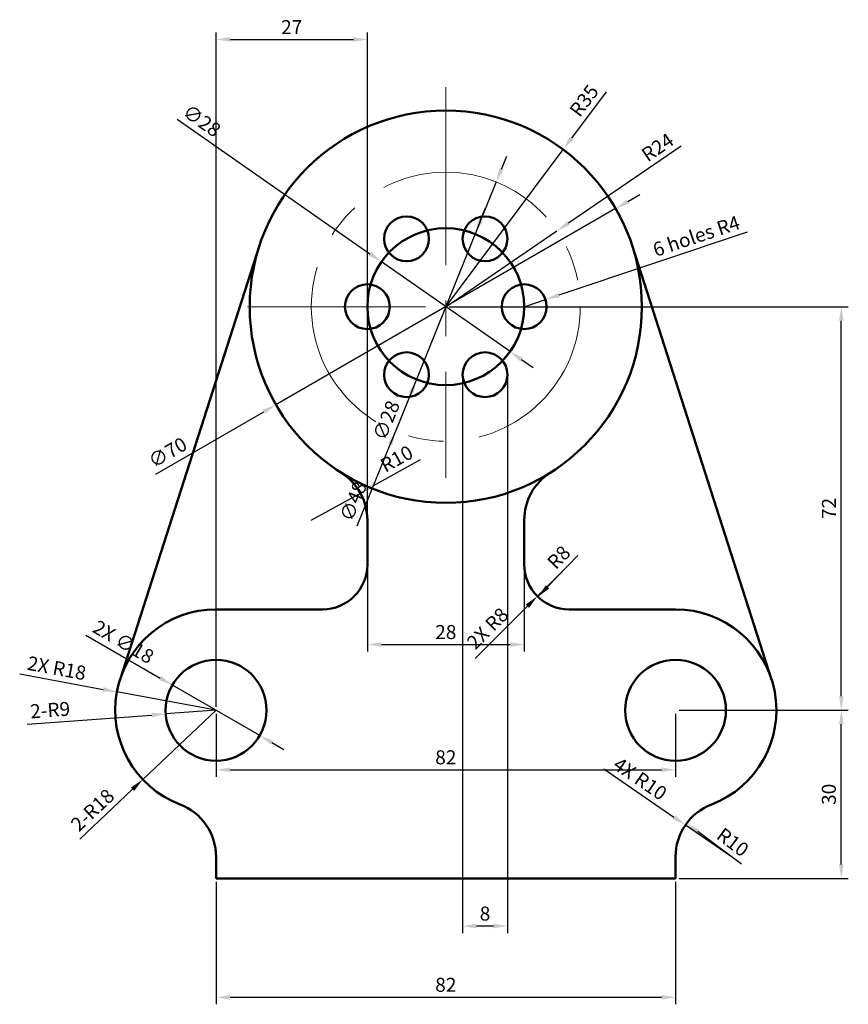
# Model space of a CAD drawing. Units: millimetres. Extents: x 2340 to 2488, y 1384 to 1560.
import ezdxf

# ---------------------------------------------------------------- set-up
doc = ezdxf.new("R2010")
doc.units = ezdxf.units.MM
doc.linetypes.add('CENTER', pattern=[50.8, 31.75, -6.35, 6.35, -6.35])
for name, color, linetype, lineweight in [('M-CNTR', 4, 'CENTER', 18), ('M-DIMS', 2, 'Continuous', 25), ('M-OUTL', 7, 'Continuous', 50)]:
    doc.layers.add(name, color=color, linetype=linetype, lineweight=lineweight)
doc.styles.get("Standard").update_dxf_attribs({"font": 'arial.ttf'})
doc.dimstyles.new('ISO-25', dxfattribs={"dimtxt": 2.5, "dimasz": 2.5, "dimexe": 1.25, "dimexo": 0.625, "dimtad": 1, "dimdec": 1, "dimdsep": 46, "dimtxsty": 'Standard', "dimcen": 2.5, "dimadec": 0, "dimazin": 0, "dimtfac": 1, "dimtdec": 1, "dimtmove": 0, "dimatfit": 3, "dimfxl": 1, "dimarcsym": 0})

# ---------------------------------------------------------------- blocks, each defined once
blk = doc.blocks.new('*U1')
blk.add_circle((0, 0), 4)
blk = doc.blocks.new('*U2')
at = {"layer": 'M-OUTL', "color": 0, "linetype": 'ByBlock', "lineweight": -2, "transparency": 16777216}
for p, rotation in [((2408.96, 1520.78), 300), ((2422.96, 1520.78), 239.9999999999999), ((2429.96, 1508.66), 180), ((2408.96, 1496.53), 59.99999999999999), ((2422.96, 1496.53), 119.9999999999999)]:
    blk.add_blockref('*U1', p, dxfattribs=dict(at, rotation=rotation))
blk.add_blockref('*U1', (2401.96, 1508.66), dxfattribs=at)
blk = doc.blocks.new('*D3')
at = {"layer": 'Defpoints', "color": 0, "lineweight": 100, "transparency": 16777216}
for p in [(2374.96, 1436.66), (2456.96, 1436.66), (2456.96, 1426.04)]:
    blk.add_point(p, dxfattribs=at)
at = {"layer": 'M-DIMS', "color": 0, "lineweight": -2, "transparency": 16777216}
for p, q in [((2374.96, 1436.03), (2374.96, 1424.79)), ((2456.96, 1436.03), (2456.96, 1424.79)), ((2377.46, 1426.04), (2454.46, 1426.04))]:
    blk.add_line(p, q, dxfattribs=at)
at = {"layer": 'M-DIMS', "color": 0, "lineweight": 100, "transparency": 16777216}
for points in [[(2377.46, 1426.46), (2377.46, 1425.63), (2374.96, 1426.04)], [(2454.46, 1426.46), (2454.46, 1425.63), (2456.96, 1426.04)]]:
    blk.add_solid(points, dxfattribs=at)
at = {"layer": 'M-DIMS', "color": 0, "transparency": 16777216, "insert": (2415.96, 1427.94), "char_height": 2.5, "attachment_point": 5}
blk.add_mtext('82', dxfattribs=at)
blk = doc.blocks.new('*D4')
at = {"layer": 'Defpoints', "color": 0, "lineweight": 100, "transparency": 16777216}
for p in [(2374.96, 1406.66), (2456.96, 1406.66), (2456.96, 1385.45)]:
    blk.add_point(p, dxfattribs=at)
at = {"layer": 'M-DIMS', "color": 0, "lineweight": -2, "transparency": 16777216}
for p, q in [((2374.96, 1406.03), (2374.96, 1384.2)), ((2456.96, 1406.03), (2456.96, 1384.2)), ((2377.46, 1385.45), (2454.46, 1385.45))]:
    blk.add_line(p, q, dxfattribs=at)
at = {"layer": 'M-DIMS', "color": 0, "lineweight": 100, "transparency": 16777216}
for points in [[(2377.46, 1385.86), (2377.46, 1385.03), (2374.96, 1385.45)], [(2454.46, 1385.86), (2454.46, 1385.03), (2456.96, 1385.45)]]:
    blk.add_solid(points, dxfattribs=at)
at = {"layer": 'M-DIMS', "color": 0, "transparency": 16777216, "insert": (2415.96, 1387.35), "char_height": 2.5, "attachment_point": 5}
blk.add_mtext('82', dxfattribs=at)
blk = doc.blocks.new('*D5')
at = {"layer": 'Defpoints', "color": 0, "lineweight": 100, "transparency": 16777216}
for p in [(2374.96, 1436.66), (2361.88, 1424.29)]:
    blk.add_point(p, dxfattribs=at)
at = {"layer": 'M-DIMS', "color": 0, "lineweight": -2, "transparency": 16777216}
for p, q in [((2374.96, 1436.66), (2361.88, 1424.29)), ((2350.62, 1413.64), (2360.07, 1422.57))]:
    blk.add_line(p, q, dxfattribs=at)
at = {"layer": 'M-DIMS', "color": 0, "lineweight": 100, "transparency": 16777216}
blk.add_solid([(2359.78, 1422.88), (2360.35, 1422.27), (2361.88, 1424.29)], dxfattribs=at)
at = {"layer": 'M-DIMS', "color": 0, "transparency": 16777216, "insert": (2353.13, 1418.63), "char_height": 2.5, "attachment_point": 5, "rotation": 43.3974}
blk.add_mtext('2-R18', dxfattribs=at)
blk = doc.blocks.new('*D6')
at = {"layer": 'Defpoints', "color": 0, "lineweight": 100, "transparency": 16777216}
for p in [(2365.99, 1436), (2374.96, 1436.66)]:
    blk.add_point(p, dxfattribs=at)
at = {"layer": 'M-DIMS', "color": 0, "lineweight": -2, "transparency": 16777216}
for p, q in [((2341.24, 1434.17), (2363.49, 1435.81)), ((2374.96, 1436.66), (2365.99, 1436))]:
    blk.add_line(p, q, dxfattribs=at)
at = {"layer": 'M-DIMS', "color": 0, "lineweight": 100, "transparency": 16777216}
blk.add_solid([(2363.46, 1436.23), (2363.52, 1435.4), (2365.99, 1436)], dxfattribs=at)
at = {"layer": 'M-DIMS', "color": 0, "transparency": 16777216, "insert": (2345.37, 1436.38), "char_height": 2.5, "attachment_point": 5, "rotation": 4.2165}
blk.add_mtext('2-R9', dxfattribs=at)
blk = doc.blocks.new('*D7')
at = {"layer": 'Defpoints', "color": 0, "lineweight": 100, "transparency": 16777216}
for p in [(2458.96, 1416.5), (2466.96, 1410.51)]:
    blk.add_point(p, dxfattribs=at)
at = {"layer": 'M-DIMS', "color": 0, "lineweight": -2, "transparency": 16777216}
blk.add_line((2468.74, 1409.18), (2460.96, 1415), dxfattribs=at)
at = {"layer": 'M-DIMS', "color": 0, "lineweight": 100, "transparency": 16777216}
blk.add_solid([(2461.21, 1415.33), (2460.71, 1414.67), (2458.96, 1416.5)], dxfattribs=at)
at = {"layer": 'M-DIMS', "color": 0, "transparency": 16777216, "insert": (2466.99, 1412.86), "char_height": 2.5, "attachment_point": 5, "rotation": 323.1905}
blk.add_mtext('R10', dxfattribs=at)
blk = doc.blocks.new('*D8')
at = {"layer": 'Defpoints', "color": 0, "lineweight": 100, "transparency": 16777216}
for p in [(2437.96, 1462.66), (2432.41, 1456.9)]:
    blk.add_point(p, dxfattribs=at)
at = {"layer": 'M-DIMS', "color": 0, "lineweight": -2, "transparency": 16777216}
blk.add_line((2439.55, 1464.3), (2434.14, 1458.7), dxfattribs=at)
at = {"layer": 'M-DIMS', "color": 0, "lineweight": 100, "transparency": 16777216}
blk.add_solid([(2433.84, 1458.99), (2434.44, 1458.41), (2432.41, 1456.9)], dxfattribs=at)
at = {"layer": 'M-DIMS', "color": 0, "transparency": 16777216, "insert": (2436.35, 1463.72), "char_height": 2.5, "attachment_point": 5, "rotation": 46.046}
blk.add_mtext('R8', dxfattribs=at)
blk = doc.blocks.new('*D9')
at = {"layer": 'Defpoints', "color": 0, "lineweight": 100, "transparency": 16777216}
for p in [(2400.72, 1475.42), (2391.96, 1470.59)]:
    blk.add_point(p, dxfattribs=at)
at = {"layer": 'M-DIMS', "color": 0, "lineweight": -2, "transparency": 16777216}
for p, q in [((2411.41, 1481.32), (2402.91, 1476.63)), ((2391.96, 1470.59), (2400.72, 1475.42))]:
    blk.add_line(p, q, dxfattribs=at)
at = {"layer": 'M-DIMS', "color": 0, "lineweight": 100, "transparency": 16777216}
blk.add_solid([(2402.71, 1477), (2403.11, 1476.27), (2400.72, 1475.42)], dxfattribs=at)
at = {"layer": 'M-DIMS', "color": 0, "transparency": 16777216, "insert": (2407.34, 1481.25), "char_height": 2.5, "attachment_point": 5, "rotation": 28.8845}
blk.add_mtext('R10', dxfattribs=at)
blk = doc.blocks.new('*D10')
at = {"layer": 'Defpoints', "color": 0, "lineweight": 100, "transparency": 16777216}
for p in [(2456.96, 1436.66), (2486.55, 1436.66), (2456.96, 1406.66)]:
    blk.add_point(p, dxfattribs=at)
at = {"layer": 'M-DIMS', "color": 0, "lineweight": -2, "transparency": 16777216}
for p, q in [((2457.59, 1436.66), (2487.8, 1436.66)), ((2486.55, 1409.16), (2486.55, 1434.16)), ((2457.59, 1406.66), (2487.8, 1406.66))]:
    blk.add_line(p, q, dxfattribs=at)
at = {"layer": 'M-DIMS', "color": 0, "lineweight": 100, "transparency": 16777216}
for points in [[(2486.13, 1434.16), (2486.96, 1434.16), (2486.55, 1436.66)], [(2486.13, 1409.16), (2486.96, 1409.16), (2486.55, 1406.66)]]:
    blk.add_solid(points, dxfattribs=at)
at = {"layer": 'M-DIMS', "color": 0, "transparency": 16777216, "insert": (2484.65, 1421.66), "char_height": 2.5, "attachment_point": 5, "rotation": 90}
blk.add_mtext('30', dxfattribs=at)
blk = doc.blocks.new('*D11')
at = {"layer": 'Defpoints', "color": 0, "lineweight": 100, "transparency": 16777216}
for p in [(2415.96, 1508.66), (2486.55, 1508.66), (2456.96, 1436.66)]:
    blk.add_point(p, dxfattribs=at)
at = {"layer": 'M-DIMS', "color": 0, "lineweight": -2, "transparency": 16777216}
for p, q in [((2416.59, 1508.66), (2487.8, 1508.66)), ((2486.55, 1439.16), (2486.55, 1506.16)), ((2457.59, 1436.66), (2487.8, 1436.66))]:
    blk.add_line(p, q, dxfattribs=at)
at = {"layer": 'M-DIMS', "color": 0, "lineweight": 100, "transparency": 16777216}
for points in [[(2486.13, 1506.16), (2486.96, 1506.16), (2486.55, 1508.66)], [(2486.13, 1439.16), (2486.96, 1439.16), (2486.55, 1436.66)]]:
    blk.add_solid(points, dxfattribs=at)
at = {"layer": 'M-DIMS', "color": 0, "transparency": 16777216, "insert": (2484.67, 1472.66), "char_height": 2.5, "attachment_point": 5, "rotation": 90}
blk.add_mtext('72', dxfattribs=at)
blk = doc.blocks.new('*D12')
at = {"layer": 'Defpoints', "color": 0, "lineweight": 100, "transparency": 16777216}
for p in [(2404.48, 1516.67), (2427.44, 1500.65)]:
    blk.add_point(p, dxfattribs=at)
at = {"layer": 'M-DIMS', "color": 0, "lineweight": -2, "transparency": 16777216}
for p, q in [((2368, 1542.13), (2402.43, 1518.1)), ((2427.44, 1500.65), (2404.48, 1516.67)), ((2429.49, 1499.22), (2431.54, 1497.79))]:
    blk.add_line(p, q, dxfattribs=at)
at = {"layer": 'M-DIMS', "color": 0, "lineweight": 100, "transparency": 16777216}
for points in [[(2402.67, 1518.44), (2402.19, 1517.76), (2404.48, 1516.67)], [(2429.73, 1499.56), (2429.25, 1498.87), (2427.44, 1500.65)]]:
    blk.add_solid(points, dxfattribs=at)
at = {"layer": 'M-DIMS', "color": 0, "transparency": 16777216, "insert": (2372.23, 1541.58), "char_height": 2.5, "attachment_point": 5, "rotation": 325.0927}
blk.add_mtext('∅28', dxfattribs=at)
blk = doc.blocks.new('*D13')
at = {"layer": 'Defpoints', "color": 0, "lineweight": 100, "transparency": 16777216}
for p in [(2435.79, 1522.18), (2415.96, 1508.66)]:
    blk.add_point(p, dxfattribs=at)
at = {"layer": 'M-DIMS', "color": 0, "lineweight": -2, "transparency": 16777216}
for p, q in [((2457.98, 1537.31), (2437.86, 1523.59)), ((2415.96, 1508.66), (2435.79, 1522.18))]:
    blk.add_line(p, q, dxfattribs=at)
at = {"layer": 'M-DIMS', "color": 0, "lineweight": 100, "transparency": 16777216}
blk.add_solid([(2437.62, 1523.93), (2438.09, 1523.24), (2435.79, 1522.18)], dxfattribs=at)
at = {"layer": 'M-DIMS', "color": 0, "transparency": 16777216, "insert": (2453.94, 1536.83), "char_height": 2.5, "attachment_point": 5, "rotation": 34.2886}
blk.add_mtext('R24', dxfattribs=at)
blk = doc.blocks.new('*D14')
at = {"layer": 'Defpoints', "color": 0, "lineweight": 100, "transparency": 16777216}
for p in [(2436.9, 1536.7), (2415.96, 1508.66)]:
    blk.add_point(p, dxfattribs=at)
at = {"layer": 'M-DIMS', "color": 0, "lineweight": -2, "transparency": 16777216}
for p, q in [((2444.59, 1546.99), (2438.4, 1538.7)), ((2415.96, 1508.66), (2436.9, 1536.7))]:
    blk.add_line(p, q, dxfattribs=at)
at = {"layer": 'M-DIMS', "color": 0, "lineweight": 100, "transparency": 16777216}
blk.add_solid([(2438.07, 1538.95), (2438.73, 1538.45), (2436.9, 1536.7)], dxfattribs=at)
at = {"layer": 'M-DIMS', "color": 0, "transparency": 16777216, "insert": (2440.9, 1545.23), "char_height": 2.5, "attachment_point": 5, "rotation": 53.2464}
blk.add_mtext('R35', dxfattribs=at)
blk = doc.blocks.new('*D15')
at = {"layer": 'Defpoints', "color": 0, "lineweight": 100, "transparency": 16777216}
for p in [(2433.76, 1509.93), (2429.96, 1508.66)]:
    blk.add_point(p, dxfattribs=at)
at = {"layer": 'M-DIMS', "color": 0, "lineweight": -2, "transparency": 16777216}
for p, q in [((2469.75, 1521.94), (2436.13, 1510.72)), ((2429.96, 1508.66), (2433.76, 1509.93))]:
    blk.add_line(p, q, dxfattribs=at)
at = {"layer": 'M-DIMS', "color": 0, "lineweight": 100, "transparency": 16777216}
blk.add_solid([(2436, 1511.11), (2436.26, 1510.32), (2433.76, 1509.93)], dxfattribs=at)
at = {"layer": 'M-DIMS', "color": 0, "transparency": 16777216, "insert": (2460.78, 1520.95), "char_height": 2.5, "attachment_point": 5, "rotation": 18.465}
blk.add_mtext('6 holes R4', dxfattribs=at)
blk = doc.blocks.new('*D16')
at = {"layer": 'Defpoints', "color": 0, "lineweight": 100, "transparency": 16777216}
for p in [(2401.96, 1466.63), (2429.96, 1466.63), (2429.96, 1448.39)]:
    blk.add_point(p, dxfattribs=at)
at = {"layer": 'M-DIMS', "color": 0, "lineweight": -2, "transparency": 16777216}
for p, q in [((2401.96, 1466), (2401.96, 1447.14)), ((2429.96, 1466), (2429.96, 1447.14)), ((2404.46, 1448.39), (2427.46, 1448.39))]:
    blk.add_line(p, q, dxfattribs=at)
at = {"layer": 'M-DIMS', "color": 0, "lineweight": 100, "transparency": 16777216}
for points in [[(2404.46, 1448.81), (2404.46, 1447.98), (2401.96, 1448.39)], [(2427.46, 1448.81), (2427.46, 1447.98), (2429.96, 1448.39)]]:
    blk.add_solid(points, dxfattribs=at)
at = {"layer": 'M-DIMS', "color": 0, "transparency": 16777216, "insert": (2415.96, 1450.29), "char_height": 2.5, "attachment_point": 5}
blk.add_mtext('28', dxfattribs=at)
blk = doc.blocks.new('MOUNTING-HOLE-D18')
blk.add_circle((9, 9), 9)
blk = doc.blocks.new('*D18')
at = {"layer": 'Defpoints', "color": 0, "lineweight": 100, "transparency": 16777216}
for p in [(2418.96, 1496.53), (2426.96, 1496.53), (2418.96, 1398.16)]:
    blk.add_point(p, dxfattribs=at)
at = {"layer": 'M-DIMS', "color": 0, "lineweight": -2, "transparency": 16777216}
for p, q in [((2418.96, 1495.91), (2418.96, 1396.91)), ((2426.96, 1495.91), (2426.96, 1396.91)), ((2424.46, 1398.16), (2421.46, 1398.16))]:
    blk.add_line(p, q, dxfattribs=at)
at = {"layer": 'M-DIMS', "color": 0, "lineweight": 100, "transparency": 16777216}
for points in [[(2421.46, 1398.58), (2421.46, 1397.74), (2418.96, 1398.16)], [(2424.46, 1398.58), (2424.46, 1397.74), (2426.96, 1398.16)]]:
    blk.add_solid(points, dxfattribs=at)
at = {"layer": 'M-DIMS', "color": 0, "transparency": 16777216, "insert": (2422.96, 1400.06), "char_height": 2.5, "attachment_point": 5}
blk.add_mtext('8', dxfattribs=at)
blk = doc.blocks.new('*D19')
at = {"layer": 'Defpoints', "color": 0, "lineweight": 100, "transparency": 16777216}
for p in [(2401.96, 1556.34), (2401.96, 1462.66), (2374.96, 1436.66)]:
    blk.add_point(p, dxfattribs=at)
at = {"layer": 'M-DIMS', "color": 0, "lineweight": -2, "transparency": 16777216}
for p, q in [((2374.96, 1437.28), (2374.96, 1557.59)), ((2401.96, 1463.28), (2401.96, 1557.59)), ((2377.46, 1556.34), (2399.46, 1556.34))]:
    blk.add_line(p, q, dxfattribs=at)
at = {"layer": 'M-DIMS', "color": 0, "lineweight": 100, "transparency": 16777216}
for points in [[(2377.46, 1556.76), (2377.46, 1555.93), (2374.96, 1556.34)], [(2399.46, 1556.76), (2399.46, 1555.93), (2401.96, 1556.34)]]:
    blk.add_solid(points, dxfattribs=at)
at = {"layer": 'M-DIMS', "color": 0, "transparency": 16777216, "insert": (2388.46, 1558.22), "char_height": 2.5, "attachment_point": 5}
blk.add_mtext('27', dxfattribs=at)
blk = doc.blocks.new('*D20')
at = {"layer": 'Defpoints', "color": 0, "lineweight": 100, "transparency": 16777216}
for p in [(2446.27, 1526.16), (2385.65, 1491.16)]:
    blk.add_point(p, dxfattribs=at)
at = {"layer": 'M-DIMS', "color": 0, "lineweight": -2, "transparency": 16777216}
for p, q in [((2448.44, 1527.41), (2450.6, 1528.66)), ((2446.27, 1526.16), (2385.65, 1491.16)), ((2364.2, 1478.77), (2383.49, 1489.91))]:
    blk.add_line(p, q, dxfattribs=at)
at = {"layer": 'M-DIMS', "color": 0, "lineweight": 100, "transparency": 16777216}
for points in [[(2448.23, 1527.77), (2448.65, 1527.05), (2446.27, 1526.16)], [(2383.28, 1490.27), (2383.69, 1489.55), (2385.65, 1491.16)]]:
    blk.add_solid(points, dxfattribs=at)
at = {"layer": 'M-DIMS', "color": 0, "transparency": 16777216, "insert": (2366.48, 1482.37), "char_height": 2.5, "attachment_point": 5, "rotation": 29.9989}
blk.add_mtext('∅70', dxfattribs=at)
blk = doc.blocks.new('*D21')
at = {"layer": 'Defpoints', "color": 0, "lineweight": 100, "transparency": 16777216}
for p in [(2424.96, 1530.91), (2406.96, 1486.41)]:
    blk.add_point(p, dxfattribs=at)
at = {"layer": 'M-DIMS', "color": 0, "lineweight": -2, "transparency": 16777216}
for p, q in [((2425.9, 1533.22), (2426.84, 1535.54)), ((2424.96, 1530.91), (2406.96, 1486.41)), ((2400.14, 1469.56), (2406.02, 1484.09))]:
    blk.add_line(p, q, dxfattribs=at)
at = {"layer": 'M-DIMS', "color": 0, "lineweight": 100, "transparency": 16777216}
for points in [[(2425.51, 1533.38), (2426.29, 1533.07), (2424.96, 1530.91)], [(2405.64, 1484.25), (2406.41, 1483.94), (2406.96, 1486.41)]]:
    blk.add_solid(points, dxfattribs=at)
at = {"layer": 'M-DIMS', "color": 0, "transparency": 16777216, "insert": (2399.73, 1473.8), "char_height": 2.5, "attachment_point": 5, "rotation": 67.9721}
blk.add_mtext('∅48', dxfattribs=at)
blk = doc.blocks.new('*D22')
at = {"layer": 'Defpoints', "color": 0, "lineweight": 100, "transparency": 16777216}
for p in [(2421.18, 1521.65), (2410.74, 1495.67)]:
    blk.add_point(p, dxfattribs=at)
at = {"layer": 'M-DIMS', "color": 0, "lineweight": -2, "transparency": 16777216}
for p, q in [((2422.12, 1523.97), (2423.05, 1526.29)), ((2421.18, 1521.65), (2410.74, 1495.67)), ((2406.06, 1484.02), (2409.81, 1493.35))]:
    blk.add_line(p, q, dxfattribs=at)
at = {"layer": 'M-DIMS', "color": 0, "lineweight": 100, "transparency": 16777216}
for points in [[(2421.73, 1524.12), (2422.5, 1523.81), (2421.18, 1521.65)], [(2409.42, 1493.5), (2410.19, 1493.19), (2410.74, 1495.67)]]:
    blk.add_solid(points, dxfattribs=at)
at = {"layer": 'M-DIMS', "color": 0, "transparency": 16777216, "insert": (2405.64, 1488.26), "char_height": 2.5, "attachment_point": 5, "rotation": 68.0991}
blk.add_mtext('∅28', dxfattribs=at)
blk = doc.blocks.new('*D23')
at = {"layer": 'Defpoints', "color": 0, "lineweight": 100, "transparency": 16777216}
for p in [(2367.17, 1441.16), (2382.75, 1432.16)]:
    blk.add_point(p, dxfattribs=at)
at = {"layer": 'M-DIMS', "color": 0, "lineweight": -2, "transparency": 16777216}
for p, q in [((2351.72, 1450.08), (2365, 1442.41)), ((2382.75, 1432.16), (2367.17, 1441.16)), ((2384.92, 1430.91), (2387.08, 1429.66))]:
    blk.add_line(p, q, dxfattribs=at)
at = {"layer": 'M-DIMS', "color": 0, "lineweight": 100, "transparency": 16777216}
for points in [[(2365.21, 1442.77), (2364.8, 1442.05), (2367.17, 1441.16)], [(2385.13, 1431.27), (2384.71, 1430.55), (2382.75, 1432.16)]]:
    blk.add_solid(points, dxfattribs=at)
at = {"layer": 'M-DIMS', "color": 0, "transparency": 16777216, "insert": (2358.27, 1448.58), "char_height": 2.5, "attachment_point": 5, "rotation": 329.9847}
blk.add_mtext('2X ∅18', dxfattribs=at)
blk = doc.blocks.new('*D24')
at = {"layer": 'Defpoints', "color": 0, "lineweight": 100, "transparency": 16777216}
for p in [(2357.26, 1439.93), (2374.96, 1436.66)]:
    blk.add_point(p, dxfattribs=at)
at = {"layer": 'M-DIMS', "color": 0, "lineweight": -2, "transparency": 16777216}
for p, q in [((2339.91, 1443.14), (2354.8, 1440.38)), ((2374.96, 1436.66), (2357.26, 1439.93))]:
    blk.add_line(p, q, dxfattribs=at)
at = {"layer": 'M-DIMS', "color": 0, "lineweight": 100, "transparency": 16777216}
blk.add_solid([(2354.88, 1440.79), (2354.73, 1439.97), (2357.26, 1439.93)], dxfattribs=at)
at = {"layer": 'M-DIMS', "color": 0, "transparency": 16777216, "insert": (2346.47, 1443.86), "char_height": 2.5, "attachment_point": 5, "rotation": 349.5298}
blk.add_mtext('2X R18', dxfattribs=at)
blk = doc.blocks.new('*D25')
at = {"layer": 'Defpoints', "color": 0, "lineweight": 100, "transparency": 16777216}
for p in [(2458.73, 1416.18), (2466.96, 1410.51)]:
    blk.add_point(p, dxfattribs=at)
at = {"layer": 'M-DIMS', "color": 0, "lineweight": -2, "transparency": 16777216}
for p, q in [((2444.16, 1426.21), (2456.67, 1417.59)), ((2466.96, 1410.51), (2458.73, 1416.18))]:
    blk.add_line(p, q, dxfattribs=at)
at = {"layer": 'M-DIMS', "color": 0, "lineweight": 100, "transparency": 16777216}
blk.add_solid([(2456.9, 1417.94), (2456.43, 1417.25), (2458.73, 1416.18)], dxfattribs=at)
at = {"layer": 'M-DIMS', "color": 0, "transparency": 16777216, "insert": (2450.46, 1424.18), "char_height": 2.5, "attachment_point": 5, "rotation": 325.4512}
blk.add_mtext('4X R10', dxfattribs=at)
blk = doc.blocks.new('*D26')
at = {"layer": 'Defpoints', "color": 0, "lineweight": 100, "transparency": 16777216}
for p in [(2437.96, 1462.66), (2432.3, 1457)]:
    blk.add_point(p, dxfattribs=at)
at = {"layer": 'M-DIMS', "color": 0, "lineweight": -2, "transparency": 16777216}
for p, q in [((2437.96, 1462.66), (2432.3, 1457)), ((2421.2, 1445.9), (2430.54, 1455.23))]:
    blk.add_line(p, q, dxfattribs=at)
at = {"layer": 'M-DIMS', "color": 0, "lineweight": 100, "transparency": 16777216}
blk.add_solid([(2430.24, 1455.53), (2430.83, 1454.94), (2432.3, 1457)], dxfattribs=at)
at = {"layer": 'M-DIMS', "color": 0, "transparency": 16777216, "insert": (2423.64, 1451.03), "char_height": 2.5, "attachment_point": 5, "rotation": 45.0002}
blk.add_mtext('2X R8', dxfattribs=at)

msp = doc.modelspace()

# ---------------------------------------------------------------- linework, layer by layer
at = {"layer": 'M-CNTR'}
for p, q in [((2415.96, 1547.84), (2415.96, 1478.15)), ((2380.59, 1508.66), (2460.2, 1508.66))]:
    msp.add_line(p, q, dxfattribs=at)
msp.add_circle((2415.96, 1508.66), 24, dxfattribs=at)
at = {"layer": 'M-OUTL'}
for p, q in [((2382.64, 1519.37), (2357.83, 1442.17)), ((2449.28, 1519.37), (2474.1, 1442.17)), ((2401.96, 1470.59), (2401.96, 1462.66)), ((2429.96, 1470.59), (2429.96, 1462.66)), ((2374.96, 1454.66), (2393.96, 1454.66)), ((2456.96, 1454.66), (2437.96, 1454.66)), ((2374.96, 1406.66), (2374.96, 1410.51)), ((2456.96, 1406.66), (2456.96, 1410.51)), ((2374.96, 1406.66), (2456.96, 1406.66))]:
    msp.add_line(p, q, dxfattribs=at)
for radius in [35, 14]:
    msp.add_circle((2415.96, 1508.66), radius, dxfattribs=at)
for centre, radius, start, end in [((2391.96, 1470.59), 10, 0, 57.769), ((2439.96, 1470.59), 10, 122.231, 180), ((2393.96, 1462.66), 8, 270, 0), ((2437.96, 1462.66), 8, 180, 270), ((2374.96, 1436.66), 18, 90, 249.0752), ((2456.96, 1436.66), 18, 290.9248, 90), ((2364.96, 1410.51), 10, 0, 69.0752), ((2466.96, 1410.51), 10, 110.9248, 180)]:
    msp.add_arc(centre, radius, start, end, dxfattribs=at)

# ---------------------------------------------------------------- block references
for name, p in [('*U2', (0, 0)), ('MOUNTING-HOLE-D18', (2365.96, 1427.66)), ('MOUNTING-HOLE-D18', (2447.96, 1427.66))]:
    msp.add_blockref(name, p, dxfattribs=at)

# ---------------------------------------------------------------- dimensions: what is measured, and where the dimension line sits
at = {"layer": 'M-DIMS'}
for base, p1, p2, override, picture, middle in [((2401.96, 1556.34), (2374.96, 1436.66), (2401.96, 1462.66), {"dimdec": 0, "dimlfac": 1, "dimrnd": 0, "dimzin": 0, "dimdsep": 46, "dimlunit": 2}, '*D19', (2388.46, 1558.22)), ((2418.96, 1398.16), (2426.96, 1496.53), (2418.96, 1496.53), {"dimdec": 0, "dimlfac": 1, "dimrnd": 0, "dimzin": 0, "dimdsep": 46, "dimlunit": 2}, '*D18', (2422.96, 1400.06)), ((2429.96, 1448.39), (2401.96, 1466.63), (2429.96, 1466.63), {"dimclrd": 0, "dimclre": 0, "dimclrt": 0}, '*D16', (2415.96, 1450.29)), ((2456.96, 1426.04), (2374.96, 1436.66), (2456.96, 1436.66), {"dimclrd": 0, "dimclre": 0, "dimclrt": 0}, '*D3', (2415.96, 1427.94)), ((2456.96, 1385.45), (2374.96, 1406.66), (2456.96, 1406.66), {"dimclrd": 0, "dimclre": 0, "dimclrt": 0}, '*D4', (2415.96, 1387.35))]:
    dim = msp.add_linear_dim(base=base, p1=p1, p2=p2, dimstyle='ISO-25', override=override, dxfattribs=at)
    dim.commit()
    dim.dimension.update_dxf_attribs({"geometry": picture, "text_midpoint": middle})
for center, mpoint, picture, middle in [((2415.96, 1508.66), (2436.9, 1536.7), '*D14', (2442.42, 1544.09)), ((2415.96, 1508.66), (2435.79, 1522.18), '*D13', (2455, 1535.28)), ((2437.96, 1462.66), (2432.41, 1456.9), '*D8', (2437.71, 1462.4)), ((2466.96, 1410.51), (2458.96, 1416.5), '*D7', (2465.85, 1411.34))]:
    dim = msp.add_radius_dim(center=center, mpoint=mpoint, dimstyle='ISO-25', override={"dimclrd": 0, "dimclre": 0, "dimclrt": 0}, dxfattribs=at)
    dim.commit()
    dim.dimension.update_dxf_attribs({"geometry": picture, "text_midpoint": middle, "dimtype": 164})
for p1, p2, override, picture, middle in [((2427.44, 1500.65), (2404.48, 1516.67), {"dimclrd": 0, "dimclre": 0, "dimclrt": 0}, '*D12', (2371.1, 1539.96)), ((2424.96, 1530.91), (2406.96, 1486.41), {"dimdec": 0, "dimlfac": 1, "dimrnd": 0, "dimzin": 0, "dimdsep": 46, "dimlunit": 2}, '*D21', (2401.56, 1473.06)), ((2446.27, 1526.16), (2385.65, 1491.16), {"dimdec": 0, "dimlfac": 1, "dimrnd": 0, "dimzin": 0, "dimdsep": 46, "dimlunit": 2}, '*D20', (2367.46, 1480.66)), ((2421.18, 1521.65), (2410.74, 1495.67), {"dimdec": 0, "dimlfac": 1, "dimrnd": 0, "dimzin": 0, "dimdsep": 46, "dimlunit": 2}, '*D22', (2407.47, 1487.52))]:
    dim = msp.add_diameter_dim_2p(p1=p1, p2=p2, dimstyle='ISO-25', override=override, dxfattribs=at)
    dim.commit()
    dim.dimension.update_dxf_attribs({"geometry": picture, "text_midpoint": middle, "dimtype": 163})
for center, mpoint, text, picture, middle in [((2429.96, 1508.66), (2433.76, 1509.93), '6 holes <>', '*D15', (2461.38, 1519.15)), ((2374.96, 1436.66), (2365.99, 1436), '2-<>', '*D6', (2345.51, 1434.49))]:
    dim = msp.add_radius_dim(center=center, mpoint=mpoint, text=text, dimstyle='ISO-25', override={"dimclrd": 0, "dimclre": 0, "dimclrt": 0}, dxfattribs=at)
    dim.commit()
    dim.dimension.update_dxf_attribs({"geometry": picture, "text_midpoint": middle, "dimtype": 164})
for base, p1, p2, picture, middle in [((2486.55, 1508.66), (2456.96, 1436.66), (2415.96, 1508.66), '*D11', (2484.67, 1472.66)), ((2486.55, 1436.66), (2456.96, 1406.66), (2456.96, 1436.66), '*D10', (2484.65, 1421.66))]:
    dim = msp.add_linear_dim(base=base, p1=p1, p2=p2, angle=90, dimstyle='ISO-25', override={"dimclrd": 0, "dimclre": 0, "dimclrt": 0}, dxfattribs=at)
    dim.commit()
    dim.dimension.update_dxf_attribs({"geometry": picture, "text_midpoint": middle})
dim = msp.add_radius_dim(center=(2391.96, 1470.59), mpoint=(2400.72, 1475.42), dimstyle='ISO-25', override={"dimclrd": 0, "dimclre": 0, "dimclrt": 0}, dxfattribs=at)
dim.commit()
dim.dimension.update_dxf_attribs({"geometry": '*D9', "text_midpoint": (2407.34, 1481.25)})
for center, mpoint, text, override, picture, middle in [((2437.96, 1462.66), (2432.3, 1457), '2X <>', {"dimdec": 0, "dimlfac": 1, "dimrnd": 0, "dimzin": 0, "dimdsep": 46, "dimlunit": 2}, '*D26', (2423.64, 1451.03)), ((2374.96, 1436.66), (2357.26, 1439.93), '2X <>', {"dimdec": 0, "dimlfac": 1, "dimrnd": 0, "dimzin": 0, "dimdsep": 46, "dimlunit": 2}, '*D24', (2346.47, 1443.86)), ((2374.96, 1436.66), (2361.88, 1424.29), '2-<>', {"dimclrd": 0, "dimclre": 0, "dimclrt": 0}, '*D5', (2353.13, 1418.63)), ((2466.96, 1410.51), (2458.73, 1416.18), '4X <>', {"dimdec": 0, "dimlfac": 1, "dimrnd": 0, "dimzin": 0, "dimdsep": 46, "dimlunit": 2}, '*D25', (2450.46, 1424.18))]:
    dim = msp.add_radius_dim(center=center, mpoint=mpoint, text=text, dimstyle='ISO-25', override=override, dxfattribs=at)
    dim.commit()
    dim.dimension.update_dxf_attribs({"geometry": picture, "text_midpoint": middle})
dim = msp.add_diameter_dim_2p(p1=(2382.75, 1432.16), p2=(2367.17, 1441.16), text='2X <>', dimstyle='ISO-25', override={"dimdec": 0, "dimlfac": 1, "dimrnd": 0, "dimzin": 0, "dimdsep": 46, "dimlunit": 2}, dxfattribs=at)
dim.commit()
dim.dimension.update_dxf_attribs({"geometry": '*D23', "text_midpoint": (2357.28, 1446.87)})

doc.saveas('drawing.dxf')
